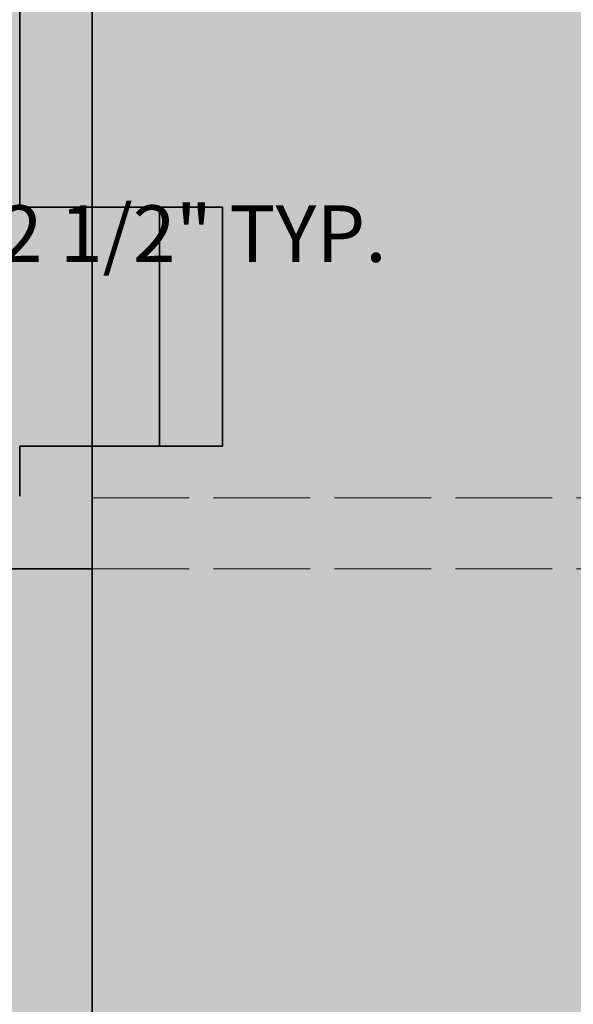
# Model space of a CAD drawing. Units: inches. Extents: x 1884 to 2398, y 474 to 1488.
# Tile 3 of 39: x 2118 to 2186, y 577 to 699. Entities that reach past the tile are written whole.
import ezdxf

# ---------------------------------------------------------------- set-up
doc = ezdxf.new("R2010")
doc.units = ezdxf.units.IN
doc.header["$MEASUREMENT"] = 0
doc.linetypes.add('ACAD_ISO02W100', pattern=[15, 12, -3])
for name, color, linetype, lineweight in [('A-ANNO-DIMS', 2, 'Continuous', 18), ('A-FLOR-OVHD', 8, 'ACAD_ISO02W100', 18), ('A-FLOR-PATT', 254, 'Continuous', 13), ('A-WALL-PATT', 250, 'Continuous', 13), ('L-TURF-PATT', 73, 'Continuous', 13), ('walls', 7, 'Continuous', 35)]:
    doc.layers.add(name, color=color, linetype=linetype, lineweight=lineweight)
doc.layers.add('L-PVMT-PATT', color=9, linetype='Continuous', lineweight=13, true_color=0xc7c8ca)
doc.styles.get("Standard").update_dxf_attribs({"font": 'arial.ttf'})
doc.dimstyles.get("Standard").update_dxf_attribs({"dimtxt": 7, "dimasz": 0.18, "dimexe": 0.18, "dimexo": 0.0625, "dimgap": 0.09, "dimtad": 0, "dimtih": 1, "dimtoh": 1, "dimzin": 0, "dimdsep": 46, "dimlunit": 3, "dimtxsty": 'Standard', "dimcen": 0.09, "dimadec": 0, "dimazin": 0, "dimtfac": 1, "dimtofl": 0, "dimtmove": 0, "dimatfit": 3, "dimfxl": 1, "dimtolj": 1, "dimtzin": 0, "dimarcsym": 0})

# ---------------------------------------------------------------- blocks, each defined once
blk = doc.blocks.new('*D29')
at = {"layer": 'A-ANNO-DIMS', "color": 0, "lineweight": -2, "transparency": 16777216}
for p, q in [((2024.65, 668.97), (2024.65, 673.08)), ((2051.26, 668.97), (2051.26, 673.08)), ((2024.83, 672.9), (2051.08, 672.9)), ((2051.26, 672.9), (2051.44, 672.9))]:
    blk.add_line(p, q, dxfattribs=at)
at = {"layer": 'A-ANNO-DIMS', "color": 0, "lineweight": 100, "transparency": 16777216}
for points in [[(2024.83, 672.93), (2024.83, 672.87), (2024.65, 672.9)], [(2051.08, 672.93), (2051.08, 672.87), (2051.26, 672.9)]]:
    blk.add_solid(points, dxfattribs=at)
at = {"layer": 'Defpoints', "color": 0, "lineweight": 100, "transparency": 16777216}
for p in [(2051.26, 672.9), (2024.65, 668.91), (2051.26, 668.91)]:
    blk.add_point(p, dxfattribs=at)
at = {"layer": 'A-ANNO-DIMS', "color": 0, "transparency": 16777216, "insert": (2108.66, 672.9), "char_height": 7, "attachment_point": 5}
blk.add_mtext('\\A1;ARMCHAIR 2\'-2 1/2" TYP.', dxfattribs=at)
blk = doc.blocks.new('*D33')
at = {"layer": 'A-ANNO-DIMS', "color": 0, "lineweight": -2, "transparency": 16777216}
for p, q in [((2021.15, 719.33), (2021.15, 724.14)), ((2052.43, 719.33), (2052.43, 724.14)), ((2021.33, 723.96), (2052.25, 723.96)), ((2052.43, 723.96), (2052.61, 723.96))]:
    blk.add_line(p, q, dxfattribs=at)
at = {"layer": 'A-ANNO-DIMS', "color": 0, "lineweight": 100, "transparency": 16777216}
for points in [[(2021.33, 723.99), (2021.33, 723.93), (2021.15, 723.96)], [(2052.25, 723.99), (2052.25, 723.93), (2052.43, 723.96)]]:
    blk.add_solid(points, dxfattribs=at)
at = {"layer": 'Defpoints', "color": 0, "lineweight": 100, "transparency": 16777216}
for p in [(2052.43, 723.96), (2021.15, 719.26), (2052.43, 719.26)]:
    blk.add_point(p, dxfattribs=at)
at = {"layer": 'A-ANNO-DIMS', "color": 0, "transparency": 16777216, "insert": (2120.18, 723.96), "char_height": 7, "attachment_point": 5}
blk.add_mtext('\\A1;COFFEE TABLE 2\'-7 1/2" TYP.', dxfattribs=at)

msp = doc.modelspace()

# ---------------------------------------------------------------- hatches: boundary and pattern name
at = {"layer": 'A-FLOR-PATT'}
h = msp.add_hatch(color=256, dxfattribs=at)
h.dxf.hatch_style = 1
h.paths.add_polyline_path([(2117.529, 815.801), (2126.529, 815.801), (2126.529, 880.382), (2117.529, 880.382), (2117.529, 892.385), (1961.529, 892.385), (1961.529, 756.915), (1964.529, 756.915), (1964.529, 759.915), (1995.529, 759.915), (1995.529, 753.915), (1972.862, 753.915), (1967.529, 756.915), (1967.529, 654.915), (1972.862, 657.915), (1995.529, 657.915), (1995.529, 651.915), (1964.529, 651.915), (1964.529, 654.915), (1961.529, 654.915), (1961.529, 640.385), (2117.529, 640.385), (2117.529, 646.578), (2126.529, 646.578), (2126.529, 676.183), (2117.529, 676.183)])
h.paths.add_polyline_path([(2012.246, 808.929), (2012.05, 810.185), (2032.542, 810.185), (2032.346, 808.929)], flags=16)
h.paths.add_polyline_path([(2010.381, 820.864), (1994.658, 820.864), (1994.658, 831.561), (1984.608, 833.132), (1984.608, 853.821), (1994.658, 855.391), (1994.658, 866.089), (2010.381, 866.089), (2011.951, 876.139), (2032.64, 876.139), (2034.211, 866.089), (2045.556, 866.089), (2047.127, 876.139), (2067.816, 876.139), (2069.386, 866.089), (2085.109, 866.089), (2085.109, 855.391), (2095.159, 853.821), (2095.159, 833.132), (2085.109, 831.561), (2085.109, 820.864), (2069.386, 820.864), (2067.816, 810.814), (2047.127, 810.814), (2045.556, 820.864), (2034.211, 820.864), (2032.64, 810.814), (2011.951, 810.814)], flags=16)
h.paths.add_polyline_path([(1982.724, 833.426), (1982.724, 853.526), (1983.98, 853.723), (1983.98, 833.23)], flags=16)
h.paths.add_polyline_path([(1994.529, 753.54), (1994.529, 658.29), (1973.529, 658.29), (1973.529, 753.54)], flags=16)
h.paths.add_polyline_path([(2084.486, 843.527), (2084.592, 843.502), (2084.681, 843.487), (2084.813, 843.477), (2084.913, 843.477), (2084.669, 843.482), (2084.336, 843.565), (2084.116, 843.617), (2083.8, 843.686), (2083.105, 843.827), (2082.836, 843.874), (2083.604, 843.729), (2084.206, 843.597)], flags=0)
h.paths.add_polyline_path([(2047.421, 808.929), (2047.225, 810.185), (2067.718, 810.185), (2067.521, 808.929)], flags=16)
h.paths.add_polyline_path([(2066.01, 849.505), (2066.429, 849.687), (2066.798, 849.882), (2067.129, 850.085), (2067.43, 850.293), (2067.711, 850.502), (2068.176, 850.856), (2068.689, 851.205), (2069.305, 851.531), (2070.015, 851.784), (2070.844, 851.944), (2071.081, 851.956), (2070.629, 851.902), (2070.212, 851.822), (2069.827, 851.717), (2069.471, 851.59), (2069.139, 851.443), (2068.828, 851.279), (2068.534, 851.1), (2068.254, 850.909), (2067.983, 850.709), (2067.502, 850.343), (2066.951, 849.962), (2066.224, 849.579)], flags=0)
h.paths.add_polyline_path([(2059.423, 853.221), (2059.827, 853.278), (2060.171, 853.358), (2060.465, 853.463), (2060.714, 853.589), (2060.926, 853.736), (2061.107, 853.902), (2061.258, 854.086), (2061.377, 854.284), (2061.462, 854.495), (2061.514, 854.715), (2061.53, 854.943), (2061.508, 855.176), (2061.449, 855.411), (2061.352, 855.646), (2061.224, 855.882), (2061.07, 856.117), (2060.9, 856.353), (2060.719, 856.588), (2060.406, 856.993), (2060.103, 857.424), (2059.858, 857.888), (2059.691, 858.467), (2059.836, 859.091), (2060.305, 859.532), (2060.844, 859.798), (2061.513, 859.935), (2062.253, 859.905), (2062.483, 859.849), (2062.078, 859.912), (2061.695, 859.928), (2061.336, 859.899), (2061.005, 859.831), (2060.703, 859.729), (2060.437, 859.597), (2060.208, 859.441), (2060.021, 859.265), (2059.879, 859.075), (2059.785, 858.874), (2059.737, 858.664), (2059.73, 858.447), (2059.761, 858.224), (2059.827, 857.996), (2059.923, 857.765), (2060.047, 857.53), (2060.193, 857.295), (2060.359, 857.06), (2060.537, 856.824), (2060.867, 856.399), (2061.171, 855.978), (2061.422, 855.518), (2061.567, 854.943), (2061.41, 854.272), (2060.947, 853.707), (2060.335, 853.397), (2059.649, 853.236)], flags=0)
h.paths.add_polyline_path([(2050.778, 859.745), (2051.07, 859.87), (2051.295, 860.017), (2051.467, 860.183), (2051.594, 860.365), (2051.679, 860.56), (2051.726, 860.763), (2051.739, 860.971), (2051.722, 861.18), (2051.677, 861.387), (2051.609, 861.587), (2051.521, 861.779), (2051.421, 861.962), (2051.312, 862.138), (2051.203, 862.307), (2050.966, 862.68), (2050.793, 863.193), (2051.021, 863.699), (2051.483, 864.018), (2052.09, 864.138), (2052.773, 864.157), (2053.007, 864.142), (2052.603, 864.152), (2052.258, 864.142), (2051.965, 864.113), (2051.716, 864.064), (2051.504, 863.995), (2051.322, 863.907), (2051.17, 863.802), (2051.048, 863.682), (2050.954, 863.55), (2050.891, 863.408), (2050.856, 863.259), (2050.851, 863.105), (2050.876, 862.948), (2050.929, 862.791), (2051.005, 862.633), (2051.098, 862.472), (2051.203, 862.307), (2051.312, 862.138), (2051.556, 861.742), (2051.751, 861.167), (2051.712, 860.535), (2051.398, 860.085), (2050.949, 859.79)], flags=0)
h.paths.add_polyline_path([(2022.768, 719.264), (2050.461, 719.264), (2050.461, 717.226), (2052.426, 717.226), (2052.426, 715.033), (2050.461, 715.033), (2050.461, 703.738), (2022.768, 703.738)], flags=16)
h.paths.add_polyline_path([(2012.246, 878.023), (2032.346, 878.023), (2032.542, 876.767), (2012.05, 876.767)], flags=16)
h.paths.add_polyline_path([(2035.324, 713.103), (2035.342, 713.294), (2035.192, 713.202)], flags=0)
h.paths.add_polyline_path([(2036.484, 711.63), (2036.583, 711.849), (2036.39, 711.898)], flags=0)
h.paths.add_polyline_path([(2036.074, 712.744), (2035.993, 712.481), (2035.724, 712.516), (2035.794, 712.726)], flags=0)
h.paths.add_polyline_path([(2035.846, 710.909), (2035.753, 710.958), (2035.702, 710.88)], flags=0)
h.paths.add_polyline_path([(2037.818, 712.019), (2037.948, 712.06), (2037.987, 712.161), (2037.815, 712.02)], flags=0)
h.paths.add_polyline_path([(2038.451, 709.517), (2038.464, 709.428), (2038.586, 709.442)], flags=0)
h.paths.add_polyline_path([(2037.805, 709.806), (2037.818, 709.807), (2037.804, 709.823)], flags=0)
h.paths.add_polyline_path([(2036.7, 711.245), (2036.698, 711.236), (2036.813, 711.211)], flags=0)
h.paths.add_polyline_path([(2035.928, 708.897), (2035.668, 708.871), (2035.706, 708.667)], flags=0)
h.paths.add_polyline_path([(2036.414, 710.976), (2035.932, 709.859), (2036.792, 710.484), (2036.5, 710.934)], flags=0)
h.paths.add_polyline_path([(2038.298, 712.115), (2038.499, 712.058), (2038.612, 712.269), (2038.39, 712.332)], flags=0)
h.paths.add_polyline_path([(2047.421, 878.023), (2067.521, 878.023), (2067.718, 876.767), (2047.225, 876.767)], flags=16)
h.paths.add_polyline_path([(2049.647, 705.093, -1), (2048.845, 705.093, -1)], flags=0)
h.paths.add_polyline_path([(2095.787, 853.723), (2097.043, 853.526), (2097.043, 833.426), (2095.787, 833.23)], flags=16)
h.paths.add_polyline_path([(2110.739, 745.339), (2111.75, 745.339, -0.0640419), (2113.267, 742.92), (2113.267, 732.192), (2113.526, 732.192, -0.4142136), (2114.278, 731.439), (2114.278, 716.764, -0.4142136), (2113.526, 716.011), (2113.267, 716.011), (2113.267, 705.284, -0.0640419), (2111.75, 702.864), (2110.739, 702.864), (2110.739, 716.011), (2109.469, 716.011, -0.4142136), (2108.716, 716.764), (2108.716, 731.439, -0.4142136), (2109.469, 732.192), (2110.739, 732.192)], flags=16)
h.paths.add_polyline_path([(1998.045, 668.909), (2002.449, 668.909), (2002.449, 652.273), (2002.724, 652.763), (2002.724, 668.175), (2019.972, 668.175), (2019.972, 652.763), (2020.247, 652.273), (2020.247, 668.909), (2024.651, 668.909), (2029.055, 668.909), (2029.055, 652.273), (2029.33, 652.763), (2029.33, 668.175), (2046.578, 668.175), (2046.578, 652.763), (2046.853, 652.273), (2046.853, 668.909), (2051.257, 668.909), (2051.257, 646.157), (2049.055, 646.157), (2049.055, 643.955), (2026.853, 643.955), (2026.853, 646.157), (2024.651, 646.157), (2022.449, 646.157), (2022.449, 643.955), (2000.247, 643.955), (2000.247, 646.157), (1998.045, 646.157)], flags=16)
h.paths.add_polyline_path([(2342.529, 1247.885), (2265.892, 1247.885), (2230.029, 1247.885), (2209.755, 1247.885), (2168.6, 1247.885), (2168.6, 1104.929), (2158.029, 1104.929), (2158.029, 1079.411), (2168.6, 1079.411), (2168.6, 1062.466), (2342.529, 1062.466), (2342.529, 1093.809)])
h.paths.add_polyline_path([(2215.03, 1153.876), (2215.03, 1164.739), (2187.559, 1164.739), (2187.442, 1152.641), (2173.568, 1152.641), (2173.684, 1164.739), (2173.684, 1218.739), (2173.801, 1230.837), (2187.675, 1230.837), (2187.559, 1218.739), (2215.03, 1218.739), (2215.03, 1225.879), (2245.053, 1225.879), (2245.053, 1153.876)], flags=16)
h.paths.add_polyline_path([(2192.147, 1164.797), (2184.963, 1174.54), (2184.915, 1174.54), (2176.755, 1174.54), (2176.755, 1190.363), (2184.915, 1190.363), (2184.915, 1196.819), (2176.755, 1196.819), (2176.755, 1212.641), (2184.915, 1212.641), (2184.915, 1174.606), (2184.963, 1174.54), (2192.147, 1174.54)], flags=0)
h.paths.add_polyline_path([(2184.971, 1158.364, -1), (2176.039, 1158.364, -1)], flags=0)
h.paths.add_polyline_path([(2335.555, 1161.985), (2335.555, 1175.132), (2334.285, 1175.132, -0.4142136), (2333.533, 1175.885), (2333.533, 1190.56, -0.4142136), (2334.285, 1191.313), (2335.555, 1191.313), (2335.555, 1204.46), (2336.567, 1204.46, -0.0640419), (2338.083, 1202.04), (2338.083, 1191.313), (2338.342, 1191.313, -0.4142136), (2339.095, 1190.56), (2339.095, 1175.885, -0.4142136), (2338.342, 1175.132), (2338.083, 1175.132), (2338.083, 1164.405, -0.0640419), (2336.567, 1161.985)], flags=16)
h.paths.add_polyline_path([(2176.155, 1224.462, -1), (2185.087, 1224.462, -1)], flags=0)
h.paths.add_polyline_path([(2158.029, 1276.197), (2158.029, 1322.885), (2148.233, 1322.885), (2092.029, 1322.885), (1961.529, 1322.885), (1961.529, 1166.885), (2116.005, 1166.885), (2116.005, 1157.885), (2152.638, 1157.885), (2152.638, 1166.885), (2158.029, 1166.885)])
h.paths.add_polyline_path([(2006.352, 1204.245), (2006.352, 1215.108), (1978.881, 1215.108), (1978.764, 1203.01), (1964.89, 1203.01), (1965.006, 1215.108), (1965.006, 1269.108), (1965.123, 1281.207), (1978.997, 1281.207), (1978.881, 1269.108), (2006.352, 1269.108), (2006.352, 1276.248), (2036.375, 1276.248), (2036.375, 1204.245)], flags=16)
h.paths.add_polyline_path([(1983.469, 1215.166), (1976.285, 1224.909), (1976.237, 1224.909), (1968.077, 1224.909), (1968.077, 1240.732), (1976.237, 1240.732), (1976.237, 1247.188), (1968.077, 1247.188), (1968.077, 1263.011), (1976.237, 1263.011), (1976.237, 1224.975), (1976.285, 1224.909), (1983.469, 1224.909)], flags=0)
h.paths.add_polyline_path([(1976.293, 1208.733, -1), (1967.361, 1208.733, -1)], flags=0)
h.paths.add_polyline_path([(1967.477, 1274.832, -1), (1976.41, 1274.832, -1)], flags=0)
h.paths.add_polyline_path([(2152.587, 1223.485), (2152.587, 1236.632), (2151.317, 1236.632, -0.4142136), (2150.564, 1237.385), (2150.564, 1252.06, -0.4142136), (2151.317, 1252.813), (2152.587, 1252.813), (2152.587, 1265.959), (2153.598, 1265.959, -0.0640419), (2155.115, 1263.54), (2155.115, 1252.813), (2155.374, 1252.813, -0.4142136), (2156.126, 1252.06), (2156.126, 1237.385, -0.4142136), (2155.374, 1236.632), (2155.115, 1236.632), (2155.115, 1225.904, -0.0640419), (2153.598, 1223.485)], flags=16)
h.paths.add_polyline_path([(2250.676, 1161.101), (2322.077, 1161.101), (2322.077, 1173.886), (2250.676, 1173.886)], flags=24)
h.paths.add_polyline_path([(2255.61, 1173.712), (2320.136, 1173.712), (2320.136, 1186.659), (2255.61, 1186.659)], flags=24)
h.paths.add_polyline_path([(2053.687, 1230.837), (2125.089, 1230.837), (2125.089, 1243.622), (2053.687, 1243.622)], flags=24)
h.paths.add_polyline_path([(2058.622, 1243.448), (2123.147, 1243.448), (2123.147, 1256.395), (2058.622, 1256.395)], flags=24)
at = {"layer": 'A-WALL-PATT'}
h = msp.add_hatch(color=256, dxfattribs=at)
h.dxf.hatch_style = 1
h.paths.add_polyline_path([(2351.529, 837.963), (2342.529, 837.963), (2342.529, 813.478), (2351.529, 813.478)])
h.paths.add_polyline_path([(2351.529, 782.175), (2342.529, 782.175), (2342.529, 778.966), (2238.447, 778.966), (2238.447, 769.966), (2351.529, 769.966)])
h.paths.add_polyline_path([(2351.529, 914.773), (2342.529, 914.773), (2342.529, 901.966), (2222.529, 901.966), (2222.529, 908.236), (2213.529, 908.236), (2213.529, 901.966), (2198.529, 901.966), (2198.529, 892.966), (2198.529, 815.857), (2203.029, 815.857), (2203.029, 892.966), (2342.529, 892.966), (2342.529, 869.555), (2346.047, 869.555), (2351.529, 869.555), (2351.529, 880.385)])
h.paths.add_polyline_path([(2208.948, 778.966), (2203.029, 778.966), (2203.029, 782.647), (2198.529, 782.647), (2198.529, 779.109), (2193.526, 779.109), (2193.526, 769.966), (2198.529, 769.966), (2208.948, 769.966)])
h.paths.add_polyline_path([(2126.529, 815.801), (2117.529, 815.801), (2117.529, 676.183), (2126.529, 676.183), (2126.529, 769.966), (2132.515, 769.966), (2132.515, 778.664), (2126.529, 778.664)])
h.paths.add_polyline_path([(2135.996, 901.385), (2009.529, 901.385), (2009.529, 929.544), (2000.529, 929.544), (2000.529, 892.385), (2117.529, 892.385), (2117.529, 880.382), (2126.529, 880.382), (2126.529, 892.385), (2135.996, 892.385)])
h.paths.add_polyline_path([(2198.529, 901.385), (2185.2, 901.385), (2185.2, 892.385), (2198.529, 892.385), (2198.529, 892.966)])
h.paths.add_polyline_path([(1961.529, 892.385), (1965.143, 892.385), (1965.143, 901.385), (1952.529, 901.385), (1952.529, 604.13), (1961.529, 604.13), (1961.529, 631.385), (1988.002, 631.385), (1988.002, 640.385), (1961.529, 640.385)])
h.paths.add_polyline_path([(1955.529, 604.13), (1952.529, 604.13), (1952.529, 530.885), (2126.529, 530.885), (2126.529, 533.885), (1955.529, 533.885)])
h.paths.add_polyline_path([(2396.529, 604.13), (2393.529, 604.13), (2393.529, 533.885), (2126.529, 533.885), (2126.529, 530.885), (2396.529, 530.885)])
h.paths.add_polyline_path([(2396.529, 779.322), (2387.529, 779.322), (2387.529, 604.13), (2396.529, 604.13)])
h = msp.add_hatch(color=256, dxfattribs=at)
h.dxf.hatch_style = 1
h.paths.add_polyline_path([(2134.868, 676.183), (2126.529, 676.183), (2126.529, 646.578), (2134.868, 646.578)])
h.paths.add_polyline_path([(2142.673, 676.183), (2134.868, 676.183), (2134.868, 646.578), (2142.673, 646.578)])
h = msp.add_hatch(color=256, dxfattribs=at)
h.dxf.hatch_style = 1
h.paths.add_polyline_path([(2126.529, 646.578), (2117.529, 646.578), (2117.529, 640.385), (2062.952, 640.385), (2062.952, 631.385), (2126.529, 631.385)])
at = {"layer": 'L-PVMT-PATT'}
h = msp.add_hatch(color=256, dxfattribs=at)
h.dxf.hatch_style = 1
h.paths.add_polyline_path([(2387.529, 769.966), (2351.529, 769.966), (2238.447, 769.966), (2238.447, 762.15), (2238.447, 754.445), (2126.529, 754.445), (2126.529, 676.183), (2134.868, 676.183), (2142.673, 676.183), (2142.673, 646.578), (2134.868, 646.578), (2126.529, 646.578), (2126.529, 640.17), (2387.529, 640.17)])
h.paths.add_polyline_path([(2387.529, 631.385), (2303.086, 631.385), (2303.086, 615.671), (2387.529, 615.671)])
h.paths.add_polyline_path([(2387.529, 640.17), (2126.529, 640.17), (2126.529, 631.385), (2387.529, 631.385)])
h.paths.add_polyline_path([(2393.529, 604.13), (2387.529, 604.13), (2387.529, 615.671), (2303.086, 615.671), (2303.086, 607.943), (2249.649, 607.943), (2126.529, 607.943), (2126.529, 533.885), (2393.529, 533.885)])
h.paths.add_polyline_path([(2257.825, 611.008), (2257.83, 611.337), (2257.915, 616.493), (2258.021, 621.805), (2258.146, 627.274), (2258.252, 631.385), (2126.529, 631.385), (2126.529, 611.008)])
h.paths.add_polyline_path([(2258.892, 611.285), (2258.888, 611.008), (2300.247, 611.008), (2300.247, 631.385), (2259.314, 631.385), (2259.206, 627.173), (2259.081, 621.72), (2258.976, 616.424)])
h = msp.add_hatch(color=256, dxfattribs=at)
h.dxf.hatch_style = 1
h.paths.add_polyline_path([(2202.48, 609.653), (2202.489, 611.008), (2126.529, 611.008), (2126.529, 607.943), (2202.484, 607.943), (2202.48, 609.055), (2202.481, 609.184)])
h.paths.add_polyline_path([(2210.813, 611.008), (2208.615, 611.008), (2208.784, 609.602), (2209.041, 607.943), (2209.165, 607.943), (2209.383, 608.672), (2210.05, 609.923)])
h.paths.add_polyline_path([(2208.179, 611.008), (2206.175, 611.008), (2206.177, 610.963), (2206.351, 608.458), (2206.392, 607.943), (2208.635, 607.943), (2208.367, 609.547)])
h.paths.add_polyline_path([(2206.177, 610.963), (2206.175, 611.008), (2204.958, 611.008), (2204.951, 610.183), (2204.925, 610.11), (2204.493, 610.081), (2204.129, 610.077), (2204.054, 610.147), (2203.949, 611.008), (2202.51, 611.008), (2202.503, 609.679), (2202.511, 607.972), (2202.537, 607.943), (2206.392, 607.943), (2206.351, 608.458)])
h.paths.add_polyline_path([(2204.425, 611.008), (2203.949, 611.008), (2204.054, 610.147), (2204.489, 610.176)], flags=17)
h.paths.add_polyline_path([(2204.958, 611.008), (2204.517, 611.008), (2204.581, 610.179), (2204.951, 610.183)], flags=17)
h.paths.add_polyline_path([(2204.517, 611.008), (2204.425, 611.008), (2204.489, 610.176), (2204.581, 610.179)], flags=17)
h.paths.add_polyline_path([(2204.489, 610.176), (2204.054, 610.147), (2204.129, 610.077), (2204.485, 610.101), (2204.561, 610.106)], flags=17)
h.paths.add_polyline_path([(2204.581, 610.179), (2204.489, 610.176), (2204.561, 610.106)], flags=17)
h.paths.add_polyline_path([(2204.951, 610.183), (2204.581, 610.179), (2204.561, 610.106), (2204.925, 610.11)], flags=17)
h.paths.add_polyline_path([(2204.925, 610.11), (2204.561, 610.106), (2204.485, 610.101), (2204.493, 610.081)], flags=17)
h.paths.add_polyline_path([(2204.485, 610.101), (2204.129, 610.077), (2204.493, 610.081)], flags=16)
at = {"layer": 'L-TURF-PATT'}
h = msp.add_hatch(color=256, dxfattribs=at)
h.dxf.hatch_style = 1
h.paths.add_polyline_path([(2126.529, 607.943), (2117.364, 607.943), (2117.364, 631.385), (1961.529, 631.385), (1961.529, 604.13), (1955.529, 604.13), (1955.529, 533.885), (2126.529, 533.885)])
h = msp.add_hatch(color=256, dxfattribs=at)
h.dxf.hatch_style = 1
h.paths.add_polyline_path([(2120.392, 631.385), (2117.364, 631.385), (2117.364, 607.943), (2126.529, 607.943), (2126.529, 611.008), (2120.392, 611.008)])
h.paths.add_polyline_path([(2126.529, 631.385), (2120.392, 631.385), (2120.392, 611.008), (2126.529, 611.008)], flags=17)

# ---------------------------------------------------------------- linework, layer by layer
at = {"layer": 'A-FLOR-OVHD'}
for p, q in [((2126.529, 640.17), (2203.428, 640.17)), ((2126.529, 631.385), (2203.439, 631.385))]:
    msp.add_line(p, q, dxfattribs=at)
at = {"layer": 'walls'}
for p, q in [((2117.529, 676.183), (2117.529, 815.801)), ((2126.529, 530.885), (2126.529, 769.966)), ((2117.529, 676.183), (2126.529, 676.183)), ((2134.868, 676.183), (2126.529, 676.183)), ((2142.673, 676.183), (2134.868, 676.183)), ((2134.868, 676.183), (2134.868, 646.578)), ((2142.673, 646.578), (2142.673, 676.183)), ((2117.529, 646.578), (2126.529, 646.578)), ((2117.529, 640.385), (2117.529, 646.578)), ((2126.529, 646.578), (2134.868, 646.578)), ((2134.868, 646.578), (2142.673, 646.578)), ((1961.529, 631.385), (2126.529, 631.385))]:
    msp.add_line(p, q, dxfattribs=at)

# ---------------------------------------------------------------- dimensions: what is measured, and where the dimension line sits
at = {"layer": 'A-ANNO-DIMS'}
for base, p1, p2, text, picture, middle in [((2052.426, 723.955), (2021.148, 719.264), (2052.426, 719.264), 'COFFEE TABLE <> TYP.', '*D33', (2120.182, 723.955)), ((2051.257, 672.9), (2024.651, 668.909), (2051.257, 668.909), 'ARMCHAIR <> TYP.', '*D29', (2108.656, 672.9))]:
    dim = msp.add_linear_dim(base=base, p1=p1, p2=p2, text=text, dimstyle='Standard', override={"dimdec": 1, "dimlfac": 1, "dimrnd": 0, "dimzin": 1, "dimdsep": 46, "dimlunit": 4, "dimfrac": 2}, dxfattribs=at)
    dim.commit()
    dim.dimension.update_dxf_attribs({"geometry": picture, "text_midpoint": middle})

doc.saveas('drawing.dxf')
